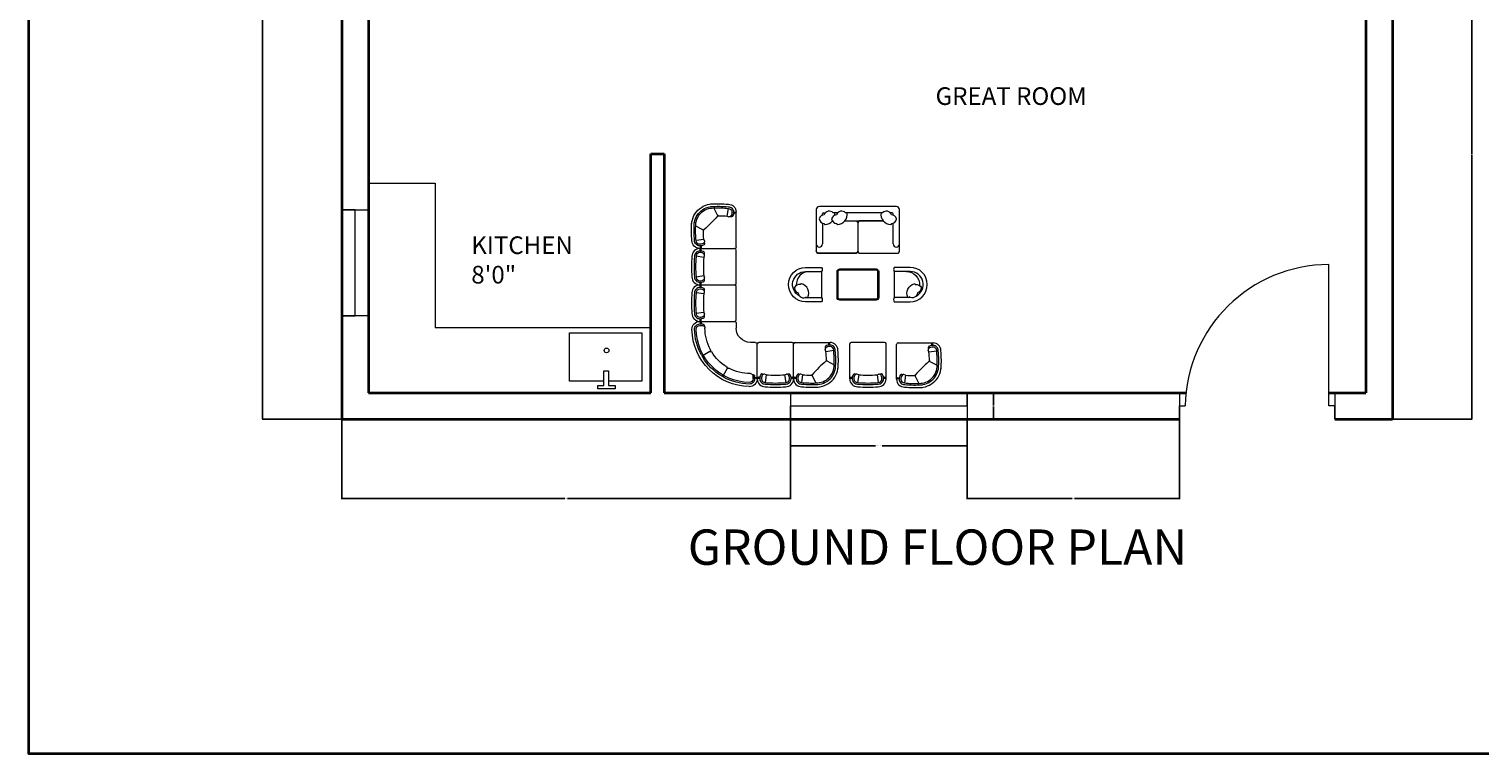
# Model space of a CAD drawing. Units: inches. Extents: x 1912 to 3731, y 1384 to 2459.
# Tile 1 of 8: x 1912 to 2405, y 1384 to 1630. Entities that reach past the tile are written whole.
import ezdxf

# ---------------------------------------------------------------- set-up
doc = ezdxf.new("R2010")
doc.units = ezdxf.units.IN
for name, color, linetype, lineweight in [('A-ANNO-DIMS', 2, 'Continuous', 18), ('A-ANNO-TITL', 7, 'Continuous', 25), ('A-ANNO-TTLB', 7, 'Continuous', 35), ('A-AREA-IDEN', 7, 'Continuous', 18), ('A-DOOR', 3, 'Continuous', 20), ('A-FLOR-CASE', 8, 'Continuous', 20), ('A-FLOR-FIXT', 9, 'Continuous', 18), ('A-FURN', 8, 'Continuous', 15), ('A-GLAZ', 4, 'Continuous', 18), ('A-WALL', 7, 'Continuous', 35)]:
    doc.layers.add(name, color=color, linetype=linetype, lineweight=lineweight)
doc.styles.get("Standard").update_dxf_attribs({"font": 'arial.ttf'})
doc.dimstyles.get("Standard").update_dxf_attribs({"dimtxt": 0.18, "dimasz": 0.18, "dimexe": 0.18, "dimexo": 0.0625, "dimgap": 0.09, "dimtad": 0, "dimtih": 1, "dimtoh": 1, "dimdec": 4, "dimzin": 0, "dimdsep": 46, "dimtxsty": 'Standard', "dimcen": 0.09, "dimadec": 0, "dimazin": 0, "dimtfac": 1, "dimtdec": 4, "dimtofl": 0, "dimtmove": 0, "dimatfit": 3, "dimfxl": 1, "dimtolj": 1, "dimtzin": 0, "dimarcsym": 0})

# ---------------------------------------------------------------- blocks, each defined once
blk = doc.blocks.new('A$C707258B2')
at = {"color": 0}
for p, q in [((0.404, 0.342), (1.074, 0.342)), ((0.404, 0.292), (0.454, 0.292)), ((1.104, 0.312), (1.104, 0.212)), ((0.404, 0.262), (0.454, 0.262)), ((0.6, -0.238), (0.47, -0.313)), ((1.479, -0.063), (1.379, -0.063)), ((1.509, -0.763), (1.509, -0.093)), ((0.929, -0.567), (0.854, -0.697)), ((1.429, -0.763), (1.429, -0.713)), ((1.459, -0.763), (1.459, -0.712))]:
    blk.add_line(p, q, dxfattribs=at)
for centre, radius, start, end in [((0.404, 0.192), 0.15, 90, 181.1754), ((0.404, 0.192), 0.1, 90, 181.1754), ((0.378, 0.317), 0.0362, 316.3972, 43.6028), ((0.368, 0.317), 0.0662, 337.8298, 22.1702), ((0.455, 0.256), 0.0357, 345.4262, 90.5555), ((1.074, 0.312), 0.03, 360, 90), ((1.379, 0.212), 1.125, 181.1754, 268.8246), ((1.379, 0.212), 1.075, 181.1754, 208.6357), ((0.404, 0.192), 0.07, 90, 181.1754), ((1.379, 0.212), 1.045, 181.1754, 268.8246), ((0.454, 0.212), 0.05, 360, 90), ((1.379, 0.212), 0.875, 180, 208.4082), ((1.379, 0.212), 0.275, 180, 270), ((0.587, -0.216), 0.025, 300, 28.4082), ((0.612, -0.259), 0.025, 31.5918, 120), ((1.379, 0.212), 0.875, 211.5918, 238.4082), ((1.479, -0.093), 0.03, 360, 90), ((0.457, -0.291), 0.025, 208.6357, 300), ((0.482, -0.334), 0.025, 120, 211.3643), ((1.379, 0.212), 1.075, 211.3643, 238.6357), ((0.907, -0.555), 0.025, 330, 58.4082), ((0.951, -0.58), 0.025, 61.5918, 150), ((0.832, -0.685), 0.025, 238.6357, 330), ((0.876, -0.71), 0.025, 150, 241.3643), ((1.379, 0.212), 1.075, 241.3643, 268.8246), ((1.379, 0.212), 0.875, 241.5918, 270), ((1.359, -0.763), 0.15, 268.8246, 360), ((1.359, -0.763), 0.1, 268.8246, 360), ((1.359, -0.763), 0.07, 268.8246, 360), ((1.379, -0.713), 0.05, 360, 90), ((1.425, -0.709), 0.0336, 354.6301, 109.3883), ((1.484, -0.799), 0.0662, 67.8298, 112.1702), ((1.484, -0.789), 0.0362, 46.3972, 133.6028)]:
    blk.add_arc(centre, radius, start, end, dxfattribs=at)
blk = doc.blocks.new('A$C1352')
at = {"color": 0}
for points in [[(0.003, 0.053), (0.003, 0.553, -0.414214), (0.053, 0.603), (0.753, 0.603, -0.414214), (0.803, 0.553), (0.803, 0.053, -0.414214), (0.753, 0.003), (0.053, 0.003, -0.414214)], [(0.023, 0.053), (0.023, 0.553, -0.414214), (0.053, 0.583), (0.753, 0.583, -0.414214), (0.783, 0.553), (0.783, 0.053, -0.414214), (0.753, 0.023), (0.053, 0.023, -0.414214)]]:
    blk.add_lwpolyline(points, format="xyb", close=True, dxfattribs=at)
blk = doc.blocks.new('part 01')
at = {"color": 0}
for p, q in [((-670, 700), (0, 700)), ((-591, 527), (-579, 561)), ((30, 30), (30, 670)), ((-591, 527), (-740, 550)), ((-591, 173), (-740, 150)), ((-670, 0), (0, 0)), ((-591, 173), (-579, 139))]:
    blk.add_line(p, q, dxfattribs=at)
for centre, radius, start, end in [((-670, 550), 150, 90, 181.1754), ((-670, 550), 100, 90, 181.1754), ((-670, 550), 70, 90, 181.1754), ((-660, 518), 133, 56.0897, 95.6132), ((-696, 675), 36.2, 316.3972, 43.6028), ((-660, 518), 103, 42.0066, 95.6132), ((-706, 675), 66.2, 337.8298, 22.1702), ((-600, 607), 25, 332.9608, 56.0897), ((-625, 620), 53.2, 321.0017, 332.9608), ((-602, 570), 25, 340, 42.0066), ((0, 670), 30, 0, 90), ((1178, 350), 2008, 174.2835, 185.7165), ((1178, 350), 1958, 174.2835, 185.7165), ((1178, 350), 1928, 174.2835, 185.7165), ((1178, 350), 1778, 174.2835, 185.7165), ((-670, 150), 150, 178.8246, 270), ((-670, 150), 100, 178.8246, 270), ((-670, 150), 70, 178.8246, 270), ((-660, 182), 133, 264.3868, 303.9103), ((-660, 182), 103, 264.3868, 317.9934), ((-696, 25), 36.2, 316.3972, 43.6028), ((-706, 25), 66.2, 337.8298, 22.1702), ((-600, 93), 25, 303.9103, 27.0392), ((-602, 130), 25, 317.9934, 20), ((-625, 80), 53.2, 27.0392, 38.9983), ((0, 30), 30, 270, 0)]:
    blk.add_arc(centre, radius, start, end, dxfattribs=at)
blk = doc.blocks.new('part02')
at = {"color": 0}
for p, q in [((0, -670), (0, 0)), ((30, 30), (700, 30)), ((621, -143), (609, -109)), ((621, -143), (770, -120)), ((640, -326), (778, -399)), ((173, -591), (139, -579)), ((173, -591), (150, -740)), ((356, -610), (429, -748))]:
    blk.add_line(p, q, dxfattribs=at)
for centre, radius, start, end in [((30, 0), 30, 90, 180), ((726, 5), 56.2, 153.6122, 206.6666), ((726, 5), 36.2, 136.3972, 223.6028), ((700, -120), 150, 0, 90), ((630, -63), 25, 123.9103, 207.0392), ((655, -50), 53.2, 207.0392, 218.9983), ((632, -100), 25, 137.9934, 200), ((690, -152), 103, 84.3868, 137.9934), ((689, -151), 132, 85.4378, 123.9887), ((-1148, -320), 1778, 0.3836, 5.7165), ((700, -121), 101, 357.5006, 89.858), ((700, -120), 70, 0, 90), ((-1228, -320), 2008, 357.7349, 5.7032), ((-1148, -320), 1958, 355.8657, 5.7165), ((-1148, -320), 2008, 355.818, 5.7165), ((2220, -2190), 2454, 130.6961, 139.3039), ((439, -409), 419, 268.2181, 1.7819), ((439, -409), 369, 268.2181, 1.7819), ((439, -409), 339, 268.2181, 1.7819), ((632, -344), 20, 62, 130.6961), ((650, -308), 20, 180.3836, 242), ((25, -696), 56.2, 63.3334, 116.3878), ((25, -696), 36.2, 46.3972, 133.6028), ((150, -670), 150, 180, 271.1754), ((182, -660), 133, 146.0897, 185.6132), ((150, -670), 100, 180, 271.1754), ((93, -600), 25, 62.9608, 146.0897), ((182, -660), 103, 132.0066, 185.6132), ((150, -670), 70, 180, 270), ((80, -625), 53.2, 51.0017, 62.9608), ((130, -602), 25, 70, 132.0066), ((350, 1258), 2008, 264.2968, 272.2651), ((350, 1178), 2008, 264.2835, 274.182), ((350, 1178), 1958, 264.2835, 274.1343), ((350, 1178), 1778, 264.2835, 269.6164), ((338, -620), 20, 28, 89.6164), ((374, -602), 20, 139.3039, 208)]:
    blk.add_arc(centre, radius, start, end, dxfattribs=at)
blk = doc.blocks.new('LOUNGE-CHAIR')
blk.add_line((5.83, 1.42), (11.22, 1.41))
at = {"ltscale": 0.03}
blk.add_lwpolyline([(11.22, 1.41, -0.369229), (11.22, 0), (5.83, 0, -1), (5.84, 11.67), (11.23, 11.67, -0.369229), (11.23, 10.25)], format="xyb", close=True, dxfattribs=at)
blk.add_lwpolyline([(3.79, 1.92, -0.785087), (5.84, 10.26), (11.23, 10.25)], format="xyb")
for centre, radius, start, end in [((7.08, 5.84), 4.42, 89.9461, 183.658), ((3.71, 4.07), 1.82, 76.6403, 159.4695), ((4.33, 5.92), 0.211, 60.6238, 203.7423), ((3.5, 2.81), 3.42, 337.0143, 74.2857), ((4, 4.88), 1.99, 184.9999, 251.3534), ((5.13, 3.08), 1.77, 182.9922, 304.1401), ((5.83, 5.84), 4.42, 268.8536, 269.9461)]:
    blk.add_arc(centre, radius, start, end)
blk = doc.blocks.new('DOOR-48-ENTRY')
for p, q in [((50.83, 40.5), (50.83, 52.5)), ((50.83, 4.5), (50.83, 40.5)), ((0, 9), (0, 0)), ((52.83, 9), (52.83, 0)), ((0, 0), (0, 4.5)), ((0, 4.5), (2, 4.5)), ((52.83, 4.5), (50.83, 4.5)), ((52.83, 0), (52.83, 4.5))]:
    blk.add_line(p, q)
blk.add_arc((50.83, 3.66), 48.84, 90, 179.0137)
blk = doc.blocks.new('WIN-PLAN-60-A')
for p, q in [((0, 9), (0, 0)), ((60, 4.5), (60, 9)), ((60, 9), (60, 0)), ((0, 0), (0, 4.5)), ((0, 4.5), (60, 4.5))]:
    blk.add_line(p, q)
blk = doc.blocks.new('WIN-PLAN-36')
for p, q in [((4.5, 36), (0, 36)), ((0, 36), (9, 36)), ((4.5, 0), (4.5, 36)), ((9, 0), (0, 0)), ((0, 0), (4.5, 0))]:
    blk.add_line(p, q)
blk = doc.blocks.new('*D31')
at = {"layer": 'A-ANNO-DIMS', "color": 0, "lineweight": -2, "transparency": 16777216}
for p, q in [((2171, 1497.56), (2171, 1488.45)), ((2231, 1497.56), (2231, 1488.45)), ((2171.18, 1488.63), (2199.88, 1488.63)), ((2230.82, 1488.63), (2202.12, 1488.63))]:
    blk.add_line(p, q, dxfattribs=at)
at = {"layer": 'A-ANNO-DIMS', "color": 0, "transparency": 16777216}
for points in [[(2171.18, 1488.66), (2171.18, 1488.6), (2171, 1488.63)], [(2230.82, 1488.66), (2230.82, 1488.6), (2231, 1488.63)]]:
    blk.add_solid(points, dxfattribs=at)
at = {"layer": 'Defpoints', "color": 0, "transparency": 16777216}
for p in [(2171, 1497.63), (2231, 1497.63), (2231, 1488.63)]:
    blk.add_point(p, dxfattribs=at)
at = {"layer": 'A-ANNO-DIMS', "color": 0, "transparency": 16777216, "insert": (2201, 1488.63), "char_height": 0.18, "attachment_point": 5}
blk.add_mtext('\\A1;WINDOW 60 TYP.', dxfattribs=at)
blk = doc.blocks.new('*D32')
at = {"layer": 'A-ANNO-DIMS', "color": 0, "lineweight": -2, "transparency": 16777216}
for p, q in [((2231.07, 1506.63), (2240.18, 1506.63)), ((2240, 1506.45), (2240, 1502.31)), ((2240, 1497.81), (2240, 1501.94)), ((2231.07, 1497.63), (2240.18, 1497.63))]:
    blk.add_line(p, q, dxfattribs=at)
at = {"layer": 'A-ANNO-DIMS', "color": 0, "transparency": 16777216}
for points in [[(2239.97, 1506.45), (2240.03, 1506.45), (2240, 1506.63)], [(2239.97, 1497.81), (2240.03, 1497.81), (2240, 1497.63)]]:
    blk.add_solid(points, dxfattribs=at)
at = {"layer": 'Defpoints', "color": 0, "transparency": 16777216}
for p in [(2231, 1506.63), (2240, 1506.63), (2231, 1497.63)]:
    blk.add_point(p, dxfattribs=at)
at = {"layer": 'A-ANNO-DIMS', "color": 0, "transparency": 16777216, "insert": (2240, 1502.13), "char_height": 0.18, "attachment_point": 5}
blk.add_mtext('\\A1;9 TYP.', dxfattribs=at)
blk = doc.blocks.new('*D92')
at = {"layer": 'A-ANNO-DIMS', "color": 0, "lineweight": -2, "transparency": 16777216}
for p, q in [((2018.47, 1973.13), (1991.4, 1973.13)), ((1991.58, 1972.95), (1991.58, 1735.56)), ((1991.58, 1497.81), (1991.58, 1735.19)), ((2018.47, 1497.63), (1991.4, 1497.63))]:
    blk.add_line(p, q, dxfattribs=at)
at = {"layer": 'A-ANNO-DIMS', "color": 0, "transparency": 16777216}
for points in [[(1991.55, 1972.95), (1991.61, 1972.95), (1991.58, 1973.13)], [(1991.55, 1497.81), (1991.61, 1497.81), (1991.58, 1497.63)]]:
    blk.add_solid(points, dxfattribs=at)
at = {"layer": 'Defpoints', "color": 0, "transparency": 16777216}
for p in [(1991.58, 1973.13), (2018.53, 1973.13), (2018.53, 1497.63)]:
    blk.add_point(p, dxfattribs=at)
at = {"layer": 'A-ANNO-DIMS', "color": 0, "transparency": 16777216, "insert": (1991.58, 1735.38), "char_height": 0.18, "attachment_point": 5}
blk.add_mtext('\\A1;475.5', dxfattribs=at)
blk = doc.blocks.new('*D96')
at = {"layer": 'A-ANNO-DIMS', "color": 0, "lineweight": -2, "transparency": 16777216}
for p, q in [((2375.59, 1677.32), (2402.66, 1677.32)), ((2402.48, 1677.14), (2402.48, 1587.66)), ((2402.48, 1497.81), (2402.48, 1587.29)), ((2375.59, 1497.63), (2402.66, 1497.63))]:
    blk.add_line(p, q, dxfattribs=at)
at = {"layer": 'A-ANNO-DIMS', "color": 0, "transparency": 16777216}
for points in [[(2402.45, 1677.14), (2402.51, 1677.14), (2402.48, 1677.32)], [(2402.45, 1497.81), (2402.51, 1497.81), (2402.48, 1497.63)]]:
    blk.add_solid(points, dxfattribs=at)
at = {"layer": 'Defpoints', "color": 0, "transparency": 16777216}
for p in [(2375.53, 1677.32), (2375.53, 1497.63), (2402.48, 1497.63)]:
    blk.add_point(p, dxfattribs=at)
at = {"layer": 'A-ANNO-DIMS', "color": 0, "transparency": 16777216, "insert": (2402.48, 1587.47), "char_height": 0.18, "attachment_point": 5}
blk.add_mtext('\\A1;179.7', dxfattribs=at)
blk = doc.blocks.new('*D97')
at = {"layer": 'A-ANNO-DIMS', "color": 0, "lineweight": -2, "transparency": 16777216}
for p, q in [((2018.53, 1497.56), (2018.53, 1470.5)), ((2171, 1497.56), (2171, 1470.5)), ((2018.71, 1470.68), (2094.31, 1470.68)), ((2170.82, 1470.68), (2095.22, 1470.68))]:
    blk.add_line(p, q, dxfattribs=at)
at = {"layer": 'A-ANNO-DIMS', "color": 0, "transparency": 16777216}
for points in [[(2018.71, 1470.71), (2018.71, 1470.65), (2018.53, 1470.68)], [(2170.82, 1470.71), (2170.82, 1470.65), (2171, 1470.68)]]:
    blk.add_solid(points, dxfattribs=at)
at = {"layer": 'Defpoints', "color": 0, "transparency": 16777216}
for p in [(2018.53, 1497.63), (2171, 1497.63), (2171, 1470.68)]:
    blk.add_point(p, dxfattribs=at)
at = {"layer": 'A-ANNO-DIMS', "color": 0, "transparency": 16777216, "insert": (2094.77, 1470.68), "char_height": 0.18, "attachment_point": 5}
blk.add_mtext('\\A1;152.47', dxfattribs=at)
blk = doc.blocks.new('*D98')
at = {"layer": 'A-ANNO-DIMS', "color": 0, "lineweight": -2, "transparency": 16777216}
for p, q in [((2231, 1497.56), (2231, 1470.5)), ((2303.12, 1497.56), (2303.12, 1470.5)), ((2231.18, 1470.68), (2266.67, 1470.68)), ((2302.94, 1470.68), (2267.45, 1470.68))]:
    blk.add_line(p, q, dxfattribs=at)
at = {"layer": 'A-ANNO-DIMS', "color": 0, "transparency": 16777216}
for points in [[(2231.18, 1470.71), (2231.18, 1470.65), (2231, 1470.68)], [(2302.94, 1470.71), (2302.94, 1470.65), (2303.12, 1470.68)]]:
    blk.add_solid(points, dxfattribs=at)
at = {"layer": 'Defpoints', "color": 0, "transparency": 16777216}
for p in [(2231, 1497.63), (2303.12, 1497.63), (2303.12, 1470.68)]:
    blk.add_point(p, dxfattribs=at)
at = {"layer": 'A-ANNO-DIMS', "color": 0, "transparency": 16777216, "insert": (2267.06, 1470.68), "char_height": 0.18, "attachment_point": 5}
blk.add_mtext('\\A1;72.12', dxfattribs=at)

msp = doc.modelspace()

# ---------------------------------------------------------------- linework, layer by layer
at = {"layer": 'A-ANNO-TTLB'}
msp.add_lwpolyline([(1912.2029, 2458.5537), (3720.218, 2458.5537), (3720.218, 1383.9599), (1912.2029, 1383.9599)], close=True, dxfattribs=at)
at = {"layer": 'A-FLOR-CASE'}
for p, q in [((2027.5308, 1577.7784), (2050.2731, 1577.7784)), ((2050.2731, 1577.7784), (2050.2731, 1528.7615)), ((2050.2731, 1528.7615), (2123.5308, 1528.7615))]:
    msp.add_line(p, q, dxfattribs=at)
at = {"layer": 'A-FLOR-FIXT'}
for points in [[(2107.5311, 1510.5247), (2095.8816, 1510.5247), (2095.8816, 1526.9171), (2120.5033, 1526.9171), (2120.5033, 1510.5247), (2109.1799, 1510.5247)], [(2107.5311, 1509.0606), (2107.5311, 1514.0627), (2109.1799, 1514.0627), (2109.1799, 1509.0606)], [(2109.1799, 1509.0606), (2111.3614, 1509.0606), (2111.3614, 1507.9708), (2105.5352, 1507.9708), (2105.5352, 1509.0606), (2107.5311, 1509.0606)]]:
    msp.add_lwpolyline(points, dxfattribs=at)
msp.add_circle((2108.4743, 1520.9732), 0.8001, dxfattribs=at)
at = {"layer": 'A-FURN'}
for p, q in [((2181.8478, 1566.8987), (2181.8478, 1567.3909)), ((2182.2014, 1567.7444), (2182.8517, 1567.7444)), ((2187.0954, 1567.7444), (2185.4037, 1567.7444)), ((2186.445, 1567.7444), (2187.0954, 1567.7444)), ((2202.3305, 1567.7444), (2189.6474, 1567.7444)), ((2205.5328, 1567.7444), (2204.8825, 1567.7444)), ((2205.8863, 1566.8987), (2205.8863, 1567.3909)), ((2181.8478, 1564.2156), (2181.8478, 1557.1392)), ((2205.8863, 1557.1392), (2205.8863, 1564.2156))]:
    msp.add_line(p, q, dxfattribs=at)
at = {"layer": 'A-FURN', "ltscale": 0.03}
msp.add_lwpolyline([(2193.8758, 1554.6647, 0.41421356), (2194.5828, 1553.9576), (2207.3004, 1553.9576, 0.41421356), (2208.0074, 1554.6647), (2208.0074, 1568.8049, 0.41421356), (2206.9469, 1569.8655), (2180.7873, 1569.8655, 0.41421356), (2179.7268, 1568.8049), (2179.7268, 1554.6647, 0.41421356), (2180.4338, 1553.9576), (2193.1514, 1553.9576, 0.41421356), (2193.8584, 1554.6647)], format="xyb", dxfattribs=at)
at = {"layer": 'A-FURN'}
for points in [[(2189.5055, 1565.0047), (2192.9833, 1565.0047, -0.41421356), (2193.8671, 1564.121), (2193.8671, 1554.8414, -0.41421356), (2192.9833, 1553.9576), (2180.6106, 1553.9576, -0.41421356), (2179.7268, 1554.8414)], [(2201.8704, 1565.0047), (2194.7509, 1565.0047, 0.41421356), (2193.8671, 1564.121), (2193.8671, 1554.8414, 0.41421356), (2194.7509, 1553.9576), (2207.1236, 1553.9576, 0.41421356), (2208.0074, 1554.8414)]]:
    msp.add_lwpolyline(points, format="xyb", dxfattribs=at)
msp.add_lwpolyline([(2189.5055, 1565.0047), (2202.4723, 1565.0047)], dxfattribs=at)
for centre, radius, start, end in [((2182.5929, 1565.0497), 1.9935, 94.543938, 160.89739), ((2182.2014, 1567.3909), 0.3535, 90, 180), ((2182.2014, 1567.3909), 0.3535, 90, 180), ((2184.1277, 1566.5163), 1.771, 41.757236, 162.905096), ((2186.8365, 1565.0497), 1.9935, 94.543938, 160.89739), ((2182.617, 1567.1759), 3.4218, 354.880983, 8.88305), ((2188.3714, 1566.5163), 1.771, 41.757236, 162.905096), ((2186.8607, 1567.1759), 3.4218, 271.611631, 8.88305), ((2205.1171, 1567.1759), 3.4218, 171.11695, 268.388369), ((2203.6065, 1566.5163), 1.771, 17.094904, 138.242764), ((2205.1413, 1565.0497), 1.9935, 19.10261, 85.456062), ((2205.5328, 1567.3909), 0.3535, 0, 90), ((2182.5142, 1565.9054), 1.8164, 186.427858, 269.256998), ((2182.6576, 1563.9594), 0.2114, 142.154994, 285.27353), ((2182.617, 1567.1759), 3.4218, 271.611631, 319.375991), ((2186.7578, 1565.9054), 1.8164, 186.427858, 269.256998), ((2186.9012, 1563.9594), 0.2114, 142.154994, 285.27353), ((2205.0766, 1563.9594), 0.2114, 254.72647, 37.845006), ((2205.22, 1565.9054), 1.8164, 270.743002, 353.572142), ((2180.7873, 1557.1392), 1.0605, 180, 270), ((2180.7873, 1557.1392), 1.0605, 270, 0), ((2206.9469, 1557.1392), 1.0605, 180, 270), ((2206.9469, 1557.1392), 1.0605, 270, 0)]:
    msp.add_arc(centre, radius, start, end, dxfattribs=at)
at = {"layer": 'A-WALL'}
for p, q in [((2018.5308, 1973.1258), (2018.5308, 1497.6258)), ((2018.5308, 1973.1258), (2018.5308, 1497.6258)), ((2375.5308, 1973.1258), (2375.5308, 1497.6258)), ((2027.5308, 1839.6258), (2027.5308, 1506.6258)), ((2366.5308, 1839.6258), (2366.5308, 1506.6258)), ((2123.5308, 1506.6258), (2123.5308, 1587.7153)), ((2123.5308, 1587.7153), (2128.0308, 1587.7153)), ((2128.0308, 1587.7153), (2128.0308, 1506.6258)), ((2027.5308, 1506.6258), (2123.5308, 1506.6258)), ((2027.5308, 1506.6258), (2123.5308, 1506.6258)), ((2128.0308, 1506.6258), (2305.4041, 1506.6258)), ((2353.9519, 1506.6258), (2366.5308, 1506.6258)), ((2018.5308, 1497.6258), (2303.1185, 1497.6258)), ((2355.9519, 1497.6258), (2375.5308, 1497.6258))]:
    msp.add_line(p, q, dxfattribs=at)

# ---------------------------------------------------------------- block references
at = {"layer": 'A-DOOR'}
msp.add_blockref('DOOR-48-ENTRY', (2303.118, 1497.626), dxfattribs=at)
at = {"layer": 'A-FURN', "ltscale": 0.03}
for name, p, xscale, yscale, zscale, rotation in [('part02', (2151.9761, 1555.6026), -0.0176753547193075, 0.0176753547193075, 0.0176753547193075, 269.9999999999968), ('A$C707258B2', (2153.6196, 1504.1859), -17.67535471930751, 17.67535471930751, 17.67535471930751, 269.9999999999968), ('part 01', (2172.0376, 1523.1683), 0.0176753547193075, 0.0176753547193075, 0.0176753547193075, 90), ('part 01', (2203.4704, 1523.1683), 0.0176753547193075, 0.0176753547193075, 0.0176753547193075, 90)]:
    msp.add_blockref(name, p, dxfattribs=dict(at, xscale=xscale, yscale=yscale, zscale=zscale, rotation=rotation))
for name, p, xscale, yscale, zscale in [('part 01', (2151.9761, 1543.2298), 0.0176753547193075, 0.0176753547193075, 0.0176753547193075), ('A$C1352', (2186.7495, 1537.9969), 17.67535471930751, 17.67535471930751, 17.67535471930751), ('part 01', (2151.9761, 1530.8571), 0.0176753547193075, 0.0176753547193075, 0.0176753547193075), ('part02', (2172.0376, 1523.1683), 0.0176753547193075, 0.0176753547193075, 0.0176753547193075), ('part02', (2207.0373, 1523.0201), 0.0176753547193075, 0.0176753547193075, 0.0176753547193075)]:
    msp.add_blockref(name, p, dxfattribs=dict(at, xscale=xscale, yscale=yscale, zscale=zscale))
at = {"layer": 'A-FURN'}
msp.add_blockref('LOUNGE-CHAIR', (2170.269, 1537.52), dxfattribs=at)
at = {"layer": 'A-FURN', "extrusion": (0, 0, -1), "zscale": -1}
msp.add_blockref('LOUNGE-CHAIR', (-2217.4652, 1537.52), dxfattribs=at)
at = {"layer": 'A-GLAZ'}
for name, p in [('WIN-PLAN-36', (2018.531, 1532.687)), ('WIN-PLAN-60-A', (2171.003, 1497.626))]:
    msp.add_blockref(name, p, dxfattribs=at)

# ---------------------------------------------------------------- texts
at = {"layer": 'A-ANNO-TITL', "insert": (2136.0849, 1460.1911), "char_height": 12, "attachment_point": 1}
msp.add_mtext_dynamic_manual_height_columns('GROUND FLOOR PLAN', width=674.920707, gutter_width=12.5, heights=[0], dxfattribs=at)
at = {"layer": 'A-AREA-IDEN', "char_height": 6, "attachment_point": 1}
for s, width, insert in [('GREAT ROOM', 172.727967, (2220.274, 1610.3352)), ('KITCHEN \\P8\'0"', 146.477552, (2062.4993, 1559.7014))]:
    msp.add_mtext_dynamic_manual_height_columns(s, width=width, gutter_width=12.5, heights=[0], dxfattribs=dict(at, insert=insert))

# ---------------------------------------------------------------- dimensions: what is measured, and where the dimension line sits
at = {"layer": 'A-ANNO-DIMS'}
for base, p1, p2, picture, middle in [((1991.5808, 1973.1258), (2018.5308, 1497.6258), (2018.5308, 1973.1258), '*D92', (1991.5808, 1735.3758)), ((2402.4808, 1497.6258), (2375.5308, 1677.3213), (2375.5308, 1497.6258), '*D96', (2402.4808, 1587.4735))]:
    dim = msp.add_linear_dim(base=base, p1=p1, p2=p2, angle=90, dimstyle='Standard', override={"dimdec": 1, "dimlfac": 1, "dimrnd": 0, "dimzin": 0, "dimdsep": 46, "dimlunit": 2}, dxfattribs=at)
    dim.commit()
    dim.dimension.update_dxf_attribs({"geometry": picture, "text_midpoint": middle})
dim = msp.add_linear_dim(base=(2240.0029, 1506.6258), p1=(2231.0029, 1497.6258), p2=(2231.0029, 1506.6258), angle=90, text='<> TYP.', dimstyle='Standard', override={"dimdec": 0, "dimlfac": 1, "dimrnd": 0, "dimzin": 0, "dimdsep": 46, "dimlunit": 2}, dxfattribs=at)
dim.commit()
dim.dimension.update_dxf_attribs({"geometry": '*D32', "text_midpoint": (2240.0029, 1502.1258)})
for base, p1, p2, picture, middle in [((2171.0029, 1470.6758), (2018.5308, 1497.6258), (2171.0029, 1497.6258), '*D97', (2094.7668, 1470.6758)), ((2303.1185, 1470.6758), (2231.0029, 1497.6258), (2303.1185, 1497.6258), '*D98', (2267.0607, 1470.6758))]:
    dim = msp.add_linear_dim(base=base, p1=p1, p2=p2, dimstyle='Standard', override={"dimdec": 2, "dimlfac": 1, "dimrnd": 0, "dimzin": 0, "dimdsep": 46, "dimlunit": 2}, dxfattribs=at)
    dim.commit()
    dim.dimension.update_dxf_attribs({"geometry": picture, "text_midpoint": middle})
dim = msp.add_linear_dim(base=(2231.0029, 1488.6258), p1=(2171.0029, 1497.6258), p2=(2231.0029, 1497.6258), text='WINDOW <> TYP.', dimstyle='Standard', override={"dimdec": 0, "dimlfac": 1, "dimrnd": 0, "dimzin": 0, "dimdsep": 46, "dimlunit": 2}, dxfattribs=at)
dim.commit()
dim.dimension.update_dxf_attribs({"geometry": '*D31', "text_midpoint": (2201.0029, 1488.6258)})

doc.saveas('drawing.dxf')
